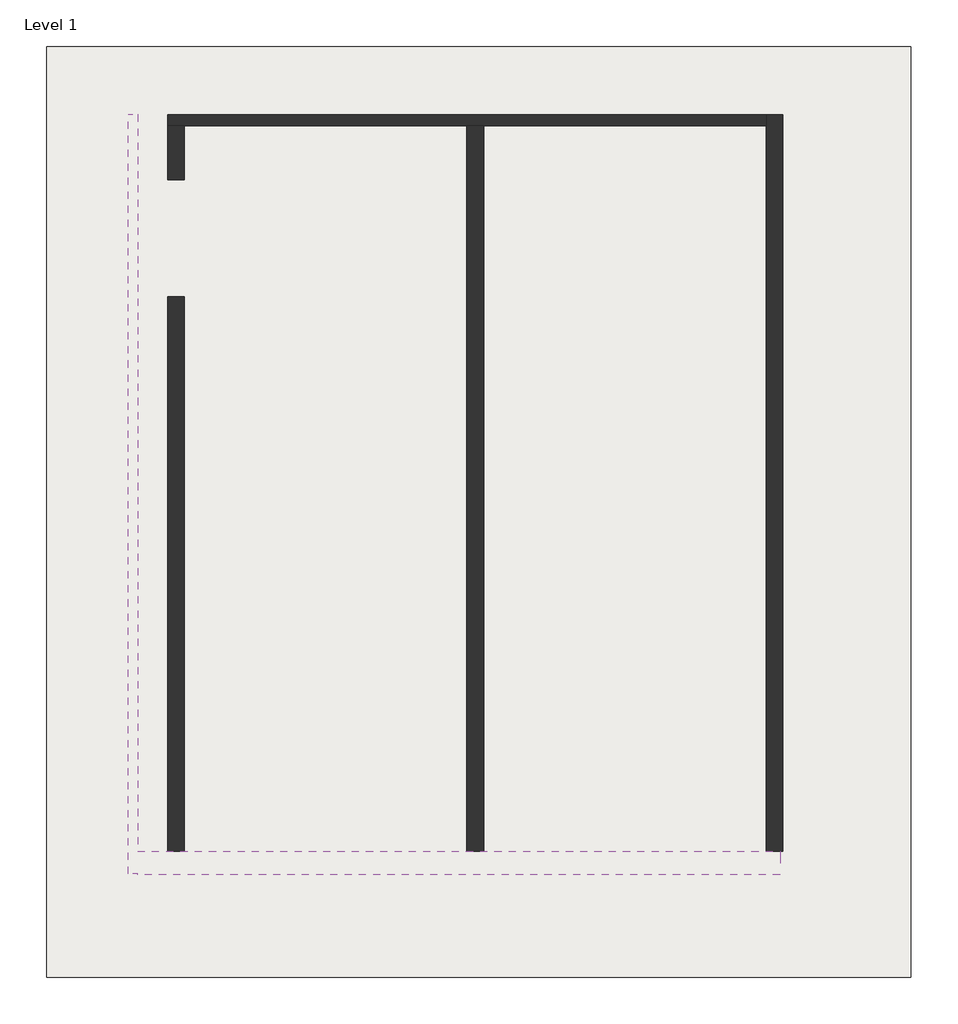
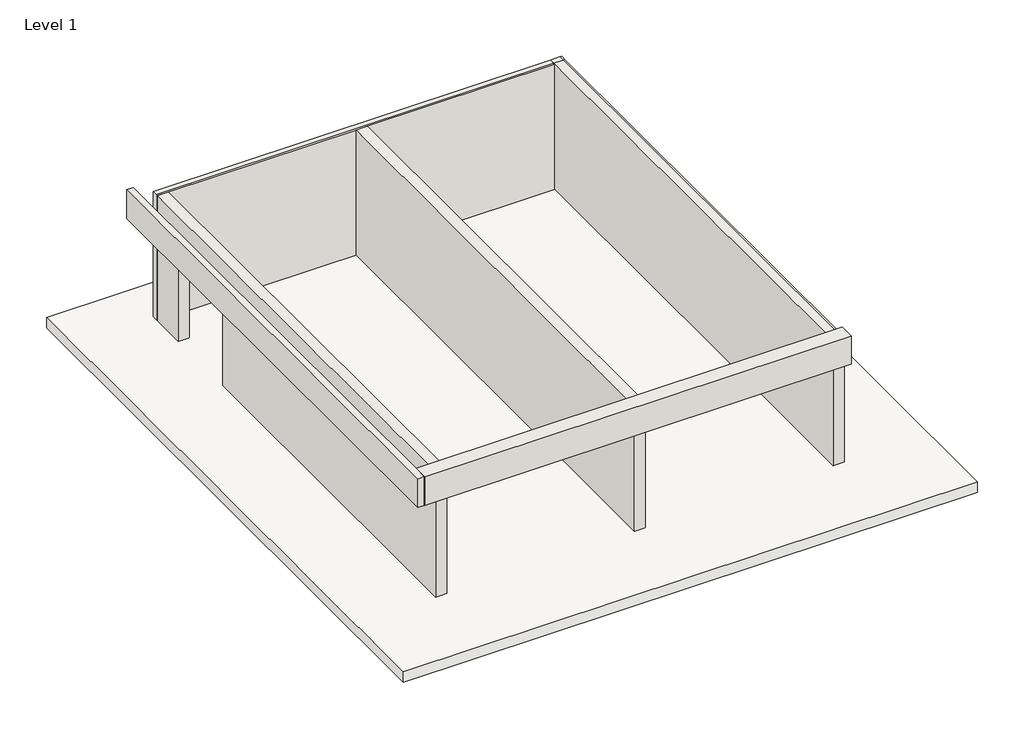
# One storey: 5 walls, 1 slab.
"""IFC4 building model written with IfcOpenShell, lengths in millimetres."""

from ifc_helpers import new_model, si_unit, frame, origin, origin_with_axes, place, context, project, spatial, polyline, outline, extrude, faceted_brep, transform, mapped, element, save
from components import walls_6_walls_6_29cd6f88

model = new_model("IFC4")

# Units and contexts
model_context = context("Model", 3, world=origin())
ifc_project = project(units=[si_unit("LENGTHUNIT", "METRE", prefix="MILLI")], contexts=[model_context])

# Site, building, storey
site = spatial("IfcSite", under=ifc_project)
building = spatial("IfcBuilding", under=site)
storey = spatial("IfcBuildingStorey", under=building, Name="Level 1", Elevation=0.0)

# Slab
placement = place(None, origin())
element("IfcSlab", 1, ObjectType="Generic - 12\"", at=placement, inside=storey, context=model_context, shape_type="SweptSolid", body=[
    extrude(outline(polyline([(5320.1690782, 10871.3734985), (5320.1690782, -6197.4265015), (-10529.4309218, -6197.4265015), (-10529.4309218, 10871.3734985), (5320.1690782, 10871.3734985)])), frame((0.0, 0.0, -304.8), z_axis=(0.0, 0.0, 1.0), x_axis=(1.0, 0.0, 0.0)), (0.0, 0.0, 1.0), 304.8),
])

# Walls
element("IfcWall", 2, ObjectType="Generic - 12\"", at=placement, inside=storey, context=model_context, shape_type="SweptSolid", body=[
    extrude(outline(polyline([(-3887.6325754, 0.0), (-3887.6325754, 3657.6), (9421.9674246, 3657.6), (9421.9674246, 0.0), (8427.7190792, 0.0), (8427.7190792, 3127.1876432), (6285.7500095, 3127.1876432), (6285.7500095, 0.0), (-3887.6325754, 0.0)])), frame((-8307.124982, 0.0, 0.0), z_axis=(1.0, 0.0, 0.0), x_axis=(0.0, 1.0, 0.0)), (0.0, 0.0, 1.0), 304.8),
])
element("IfcWall", 3, ObjectType="Generic - 12\"", at=placement, inside=storey, context=model_context, shape_type="Brep", body=[
    faceted_brep([(2665.675018, 9625.1674246, 0.0), (2665.675018, 9421.9674246, 0.0), (2665.675018, -3887.6325754, 0.0), (2665.675018, -3887.6325754, 3657.6), (2665.675018, 9421.9674246, 3657.6), (2665.675018, 9472.7674246, 3657.6), (2665.675018, 9625.1674246, 3657.6), (2970.475018, 9625.1674246, 0.0), (2970.475018, 9625.1674246, 3657.6), (2970.475018, 9472.7674246, 3657.6), (2970.475018, -3887.6325754, 3657.6), (2970.475018, -3887.6325754, 0.0), (2924.6563456, -3887.6325754, 3657.6), (2924.6563456, 9625.1674246, 3657.6), (2924.6563456, 9472.7674246, 3657.6)], [[[0, 1, 2, 3, 4, 5, 6]], [[7, 8, 9, 10, 11]], [[2, 1, 0, 7, 11]], [[3, 2, 11, 10, 12]], [[0, 6, 13, 8, 7]], [[5, 4, 3, 12, 14]], [[12, 10, 9, 14]], [[6, 5, 14, 13]], [[14, 9, 8, 13]]]),
])
element("IfcWall", 4, ObjectType="Generic - 12\"", at=placement, inside=storey, context=model_context, shape_type="SweptSolid", body=[
    extrude(outline(polyline([(-2515.924982, 9421.9674246), (-2515.924982, -3887.6325754), (-2820.724982, -3887.6325754), (-2820.724982, 9421.9674246), (-2515.924982, 9421.9674246)])), origin_with_axes(), (0.0, 0.0, 1.0), 3657.6),
])
element("IfcWall", 5, ObjectType="Generic - 8\"", at=placement, inside=storey, context=model_context, shape_type="Brep", body=[
    faceted_brep([(-8307.124982, 9421.9674246, 0.0), (-8002.324982, 9421.9674246, 0.0), (-2820.724982, 9421.9674246, 0.0), (-2515.924982, 9421.9674246, 0.0), (2665.675018, 9421.9674246, 0.0), (2665.675018, 9421.9674246, 3657.6), (-2515.924982, 9421.9674246, 3657.6), (-2820.724982, 9421.9674246, 3657.6), (-8002.324982, 9421.9674246, 3657.6), (-8307.124982, 9421.9674246, 3657.6), (-8307.124982, 9625.1674246, 0.0), (-8307.124982, 9625.1674246, 3657.6), (2665.675018, 9625.1674246, 3657.6), (2665.675018, 9625.1674246, 0.0), (-8307.124982, 9472.7674246, 3657.6), (2665.675018, 9472.7674246, 3657.6)], [[[0, 1, 2, 3, 4, 5, 6, 7, 8, 9]], [[10, 11, 12, 13]], [[4, 3, 2, 1, 0, 10, 13]], [[0, 9, 14, 11, 10]], [[5, 4, 13, 12, 15]], [[9, 8, 7, 6, 5, 15, 14]], [[15, 12, 11, 14]]]),
])
walls_6_walls_6_shape = walls_6_walls_6_29cd6f88(model_context)
element("IfcWall", 6, ObjectType="Walls 6 : Walls 6", at=placement, inside=storey, context=model_context, shape_type="MappedRepresentation", body=[
    mapped(walls_6_walls_6_shape, transform((0.0, 0.0, 0.0), x_axis=(1.0, 0.0, 0.0), y_axis=(0.0, 1.0, 0.0), z_axis=(0.0, 0.0, 1.0))),
])

save(model, "model.ifc")

# Revit data of these elements
# Type "Generic - 12\""
#   Assembly Code = "B1010"
#   Function = 0
#   Layers, outside or top first: 1' - 0" no material (function 1)
# Type "Generic - 12\""
#   Assembly Code = "B2010"
#   Layers, outside or top first: 1' - 0" no material (function 1)
# Type "Generic - 8\""
#   Assembly Code = "B2010"
#   Layers, outside or top first: 0' - 8" no material (function 1)
# Element 1 (IfcSlab, "Generic - 12\"")
#   Height Offset From Level = 0' - 0"
#   Phase Created = New Construction
#   Materials on its faces: "Default Floor"
# Elements 2, 3, 4 (IfcWall, "Generic - 12\"")
#   Top Offset = 0' - 0"
#   Base Offset = 0' - 0"
#   Unconnected Height = 12' - 0"
#   wall height = 12' - 0"
#   Phase Created = New Construction
#   Base Constraint = Level 1
#   Materials on its faces: "Default Wall"
# Element 5 (IfcWall, "Generic - 8\"")
#   Top Offset = 0' - 0"
#   Base Offset = 0' - 0"
#   Unconnected Height = 12' - 0"
#   wall height = 12' - 0"
#   Phase Created = New Construction
#   Base Constraint = Level 1
#   Materials on its faces: "Default Wall"
# Element 6 (IfcWall, "Walls 6 : Walls 6")
#   Phase Created = New Construction
#   Materials on its faces: "Default Wall"
# Materials
#   "Default Floor": colour RGB 128 128 128, transparency 0
#   "Default Wall": colour RGB 128 128 128, transparency 0
